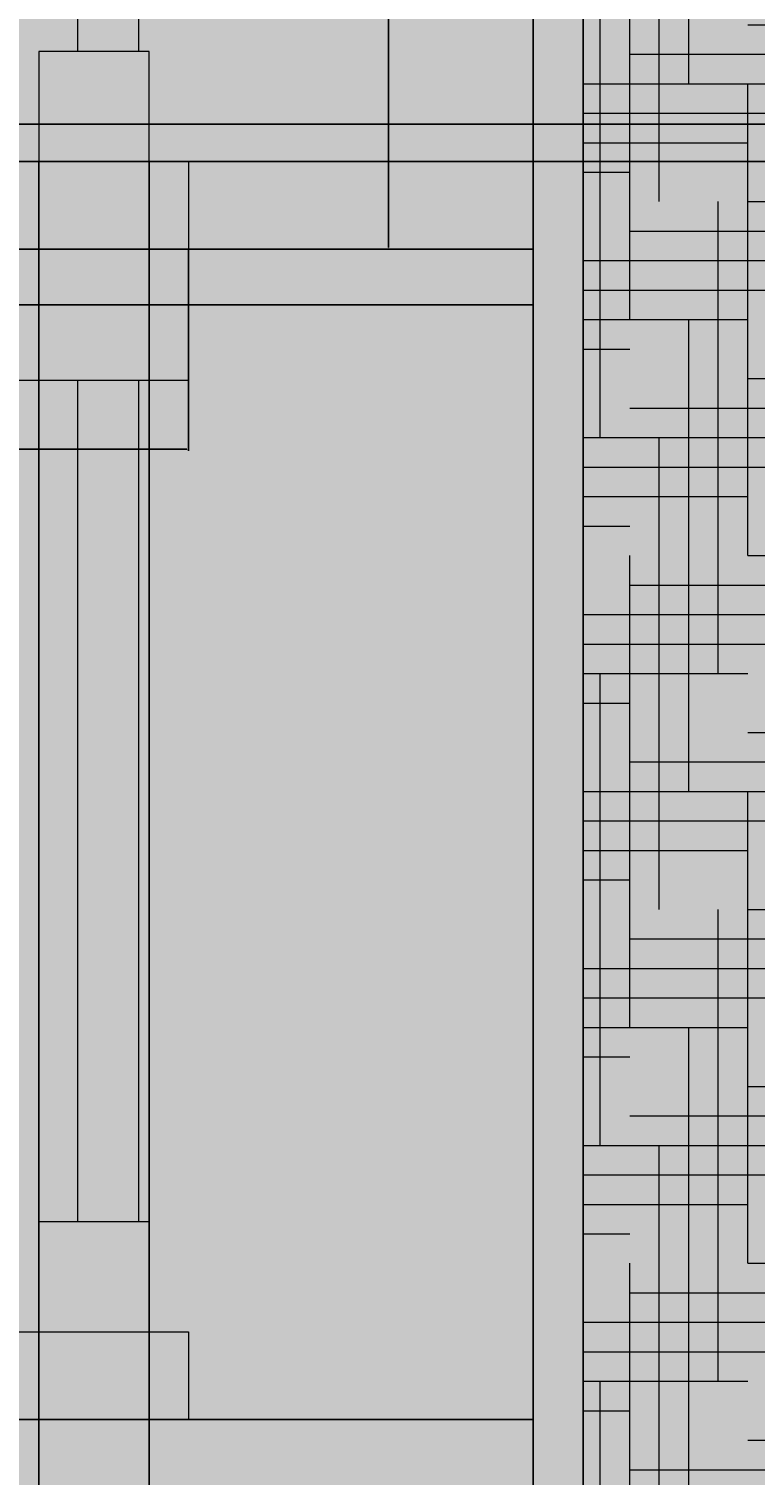
# Model space of a CAD drawing. Units: inches. Extents: x 3024 to 4744, y 1110 to 2100.
# Tile 22 of 29: x 3275 to 3354, y 1654 to 1809. Entities that reach past the tile are written whole.
import ezdxf

# ---------------------------------------------------------------- set-up
doc = ezdxf.new("R2010")
doc.units = ezdxf.units.IN
for name, color, linetype, lineweight in [('A-ANNO-DIMS', 2, 'Continuous', 18), ('A-ELEV', 7, 'Continuous', 25), ('A-ELEV-PATT', 252, 'Continuous', 13), ('A-GLAZ', 4, 'Continuous', 18)]:
    doc.layers.add(name, color=color, linetype=linetype, lineweight=lineweight)
doc.styles.get("Standard").update_dxf_attribs({"font": 'arial.ttf'})
doc.dimstyles.get("Standard").update_dxf_attribs({"dimtxt": 0.18, "dimasz": 0.18, "dimexe": 0.18, "dimexo": 0.0625, "dimgap": 0.09, "dimtad": 0, "dimtih": 1, "dimtoh": 1, "dimdec": 1, "dimzin": 0, "dimdsep": 46, "dimlunit": 3, "dimtxsty": 'Standard', "dimcen": 0.09, "dimadec": 0, "dimazin": 0, "dimtfac": 1, "dimtdec": 1, "dimtofl": 0, "dimtmove": 0, "dimatfit": 3, "dimfxl": 1, "dimtolj": 1, "dimtzin": 0, "dimarcsym": 0})

# ---------------------------------------------------------------- blocks, each defined once
blk = doc.blocks.new('WIN-BALCONY-A')
for p, q in [((3169.4, 1897.49), (3148.97, 1897.49)), ((3169.4, 1897.49), (3148.97, 1897.49)), ((3169.4, 1897.49), (3292.61, 1897.49)), ((3169.4, 1897.49), (3292.61, 1897.49)), ((3169.4, 1795.04), (3148.97, 1795.04)), ((3169.4, 1795.04), (3148.97, 1795.04)), ((3169.4, 1795.04), (3292.61, 1795.04)), ((3169.4, 1795.04), (3292.61, 1795.04))]:
    blk.add_line(p, q)
for points in [[(3148.97, 1897.49), (3148.97, 1905.61), (3292.61, 1905.61), (3292.61, 1897.49)], [(3148.97, 1897.49), (3148.97, 1905.61), (3292.61, 1905.61), (3292.61, 1897.49)], [(3292.61, 1795.04), (3292.61, 1785.61), (3148.97, 1785.61), (3148.97, 1795.04)], [(3292.61, 1795.04), (3292.61, 1785.61), (3148.97, 1785.61), (3148.97, 1795.04)]]:
    blk.add_lwpolyline(points)
for points in [[(3154.33, 1806.87), (3160.86, 1806.87), (3160.86, 1897.49), (3154.33, 1897.49)], [(3154.33, 1806.87), (3160.86, 1806.87), (3160.86, 1897.49), (3154.33, 1897.49)], [(3272.18, 1795.04), (3169.4, 1795.04), (3169.4, 1897.49), (3272.18, 1897.49)], [(3272.18, 1795.04), (3169.4, 1795.04), (3169.4, 1897.49), (3272.18, 1897.49)], [(3287.25, 1806.87), (3280.72, 1806.87), (3280.72, 1897.49), (3287.25, 1897.49)], [(3287.25, 1806.87), (3280.72, 1806.87), (3280.72, 1897.49), (3287.25, 1897.49)], [(3268.18, 1799.04), (3173.4, 1799.04), (3173.4, 1893.49), (3268.18, 1893.49)], [(3268.18, 1799.04), (3173.4, 1799.04), (3173.4, 1893.49), (3268.18, 1893.49)], [(3220.05, 1893.49), (3221.52, 1893.49), (3221.52, 1799.04), (3220.05, 1799.04)], [(3220.05, 1893.49), (3221.52, 1893.49), (3221.52, 1799.04), (3220.05, 1799.04)], [(3163.53, 1795.04), (3151.66, 1795.04), (3151.66, 1806.87), (3163.53, 1806.87)], [(3163.53, 1795.04), (3151.66, 1795.04), (3151.66, 1806.87), (3163.53, 1806.87)], [(3276.51, 1795.04), (3288.38, 1795.04), (3288.38, 1806.87), (3276.51, 1806.87)], [(3276.51, 1795.04), (3288.38, 1795.04), (3288.38, 1806.87), (3276.51, 1806.87)]]:
    blk.add_lwpolyline(points, close=True)
blk = doc.blocks.new('*D6')
at = {"layer": 'A-ANNO-DIMS', "color": 0, "lineweight": -2, "transparency": 16777216}
for p, q in [((3148.97, 1785.55), (3148.97, 1763.89)), ((3292.61, 1785.55), (3292.61, 1763.89)), ((3149.15, 1764.07), (3218.85, 1764.07)), ((3292.43, 1764.07), (3222.72, 1764.07))]:
    blk.add_line(p, q, dxfattribs=at)
at = {"layer": 'A-ANNO-DIMS', "color": 0, "transparency": 16777216}
for points in [[(3149.15, 1764.1), (3149.15, 1764.04), (3148.97, 1764.07)], [(3292.43, 1764.1), (3292.43, 1764.04), (3292.61, 1764.07)]]:
    blk.add_solid(points, dxfattribs=at)
at = {"layer": 'Defpoints', "color": 0, "transparency": 16777216}
for p in [(3148.97, 1785.61), (3292.61, 1785.61), (3292.61, 1764.07)]:
    blk.add_point(p, dxfattribs=at)
at = {"layer": 'A-ANNO-DIMS', "color": 0, "transparency": 16777216, "insert": (3220.79, 1764.07), "char_height": 0.18, "attachment_point": 5}
blk.add_mtext('\\A1;BALCONY WINDOW A 144 TYP.', dxfattribs=at)
blk = doc.blocks.new('*D7')
at = {"layer": 'A-ANNO-DIMS', "color": 0, "lineweight": -2, "transparency": 16777216}
for p, q in [((3292.67, 1905.61), (3314.33, 1905.61)), ((3314.15, 1905.43), (3314.15, 1845.79)), ((3314.15, 1785.79), (3314.15, 1845.43)), ((3292.67, 1785.61), (3314.33, 1785.61))]:
    blk.add_line(p, q, dxfattribs=at)
at = {"layer": 'A-ANNO-DIMS', "color": 0, "transparency": 16777216}
for points in [[(3314.12, 1905.43), (3314.18, 1905.43), (3314.15, 1905.61)], [(3314.12, 1785.79), (3314.18, 1785.79), (3314.15, 1785.61)]]:
    blk.add_solid(points, dxfattribs=at)
at = {"layer": 'Defpoints', "color": 0, "transparency": 16777216}
for p in [(3292.61, 1905.61), (3314.15, 1905.61), (3292.61, 1785.61)]:
    blk.add_point(p, dxfattribs=at)
at = {"layer": 'A-ANNO-DIMS', "color": 0, "transparency": 16777216, "insert": (3314.15, 1845.61), "char_height": 0.18, "attachment_point": 5}
blk.add_mtext('\\A1;120 TYP.', dxfattribs=at)
blk = doc.blocks.new('*D64')
at = {"layer": 'A-ANNO-DIMS', "color": 0, "lineweight": -2, "transparency": 16777216}
for p, q in [((3069.79, 1241.5), (3069.79, 2100.44)), ((3741.15, 1241.5), (3741.15, 2100.44)), ((3069.97, 2100.26), (3405.08, 2100.26)), ((3740.97, 2100.26), (3405.87, 2100.26))]:
    blk.add_line(p, q, dxfattribs=at)
at = {"layer": 'A-ANNO-DIMS', "color": 0, "transparency": 16777216}
for points in [[(3069.97, 2100.29), (3069.97, 2100.23), (3069.79, 2100.26)], [(3740.97, 2100.29), (3740.97, 2100.23), (3741.15, 2100.26)]]:
    blk.add_solid(points, dxfattribs=at)
at = {"layer": 'Defpoints', "color": 0, "transparency": 16777216}
for p in [(3741.15, 2100.26), (3069.79, 1241.43), (3741.15, 1241.43)]:
    blk.add_point(p, dxfattribs=at)
at = {"layer": 'A-ANNO-DIMS', "color": 0, "transparency": 16777216, "insert": (3405.47, 2100.26), "char_height": 0.18, "attachment_point": 5}
blk.add_mtext('\\A1;671.4', dxfattribs=at)
blk = doc.blocks.new('*D94')
at = {"layer": 'A-ANNO-DIMS', "color": 0, "lineweight": -2, "transparency": 16777216}
for p, q in [((3276.51, 1794.98), (3276.51, 1109.93)), ((3288.38, 1794.98), (3288.38, 1109.93)), ((3276.69, 1110.11), (3281.99, 1110.11)), ((3288.2, 1110.11), (3282.9, 1110.11))]:
    blk.add_line(p, q, dxfattribs=at)
at = {"layer": 'A-ANNO-DIMS', "color": 0, "transparency": 16777216}
for points in [[(3276.69, 1110.14), (3276.69, 1110.08), (3276.51, 1110.11)], [(3288.2, 1110.14), (3288.2, 1110.08), (3288.38, 1110.11)]]:
    blk.add_solid(points, dxfattribs=at)
at = {"layer": 'Defpoints', "color": 0, "transparency": 16777216}
for p in [(3276.51, 1795.04), (3288.38, 1795.04), (3288.38, 1110.11)]:
    blk.add_point(p, dxfattribs=at)
at = {"layer": 'A-ANNO-DIMS', "color": 0, "transparency": 16777216, "insert": (3282.44, 1110.11), "char_height": 0.18, "attachment_point": 5}
blk.add_mtext('\\A1;11.866', dxfattribs=at)
blk = doc.blocks.new('*D100')
at = {"layer": 'A-ANNO-DIMS', "color": 0, "lineweight": -2, "transparency": 16777216}
for p, q in [((3268.24, 1799.04), (3786.83, 1799.04)), ((3786.65, 1798.86), (3786.65, 1797.23)), ((3786.65, 1795.22), (3786.65, 1796.86)), ((3272.24, 1795.04), (3786.83, 1795.04))]:
    blk.add_line(p, q, dxfattribs=at)
at = {"layer": 'A-ANNO-DIMS', "color": 0, "transparency": 16777216}
for points in [[(3786.62, 1798.86), (3786.68, 1798.86), (3786.65, 1799.04)], [(3786.62, 1795.22), (3786.68, 1795.22), (3786.65, 1795.04)]]:
    blk.add_solid(points, dxfattribs=at)
at = {"layer": 'Defpoints', "color": 0, "transparency": 16777216}
for p in [(3268.18, 1799.04), (3786.65, 1799.04), (3272.18, 1795.04)]:
    blk.add_point(p, dxfattribs=at)
at = {"layer": 'A-ANNO-DIMS', "color": 0, "transparency": 16777216, "insert": (3786.65, 1797.04), "char_height": 0.18, "attachment_point": 5}
blk.add_mtext('\\A1;4.00', dxfattribs=at)
blk = doc.blocks.new('*D101')
at = {"layer": 'A-ANNO-DIMS', "color": 0, "lineweight": -2, "transparency": 16777216}
for p, q in [((3268.24, 1893.49), (3786.83, 1893.49)), ((3786.65, 1893.31), (3786.65, 1846.45)), ((3786.65, 1799.22), (3786.65, 1846.08)), ((3268.24, 1799.04), (3786.83, 1799.04))]:
    blk.add_line(p, q, dxfattribs=at)
at = {"layer": 'A-ANNO-DIMS', "color": 0, "transparency": 16777216}
for points in [[(3786.62, 1893.31), (3786.68, 1893.31), (3786.65, 1893.49)], [(3786.62, 1799.22), (3786.68, 1799.22), (3786.65, 1799.04)]]:
    blk.add_solid(points, dxfattribs=at)
at = {"layer": 'Defpoints', "color": 0, "transparency": 16777216}
for p in [(3268.18, 1893.49), (3786.65, 1893.49), (3268.18, 1799.04)]:
    blk.add_point(p, dxfattribs=at)
at = {"layer": 'A-ANNO-DIMS', "color": 0, "transparency": 16777216, "insert": (3786.65, 1846.27), "char_height": 0.18, "attachment_point": 5}
blk.add_mtext('\\A1;94.44', dxfattribs=at)

msp = doc.modelspace()

# ---------------------------------------------------------------- hatches: boundary and pattern name
at = {"layer": 'A-ELEV-PATT'}
h = msp.add_hatch(color=256, dxfattribs=at)
h.dxf.hatch_style = 1
h.paths.add_polyline_path([(3491.8271, 2054.7584), (3320.5658, 2054.7584), (3320.5658, 2043.5286), (3491.8271, 2043.5286)])
h.paths.add_polyline_path([(3292.6051, 1905.6112), (3148.9694, 1905.6112), (3148.9694, 1897.4879), (3169.3964, 1897.4879), (3292.6051, 1897.4879)])
h.paths.add_polyline_path([(3292.6051, 1795.0431), (3169.3964, 1795.0431), (3148.9694, 1795.0431), (3148.9694, 1785.6112), (3292.6051, 1785.6112)])
h.paths.add_polyline_path([(3292.6051, 1779.6112), (3148.9694, 1779.6112), (3148.9694, 1771.4879), (3169.3964, 1771.4879), (3292.6051, 1771.4879)])
h.paths.add_polyline_path([(3292.6051, 1669.0431), (3169.3964, 1669.0431), (3148.9694, 1669.0431), (3148.9694, 1659.6112), (3292.6051, 1659.6112)])
h.paths.add_polyline_path([(3292.6051, 1653.6112), (3148.9694, 1653.6112), (3148.9694, 1645.4879), (3169.3964, 1645.4879), (3292.6051, 1645.4879)])
h.paths.add_polyline_path([(3292.6051, 1543.0431), (3169.3964, 1543.0431), (3148.9694, 1543.0431), (3148.9694, 1533.6112), (3292.6051, 1533.6112)])
h.paths.add_polyline_path([(3292.6051, 1527.6112), (3148.9694, 1527.6112), (3148.9694, 1519.4879), (3169.3964, 1519.4879), (3292.6051, 1519.4879)])
h.paths.add_polyline_path([(3292.6051, 1401.6112), (3148.9694, 1401.6112), (3148.9694, 1393.4879), (3169.3964, 1393.4879), (3292.6051, 1393.4879)])
h.paths.add_polyline_path([(3292.6051, 1417.0431), (3169.3964, 1417.0431), (3148.9694, 1417.0431), (3148.9694, 1407.6112), (3292.6051, 1407.6112)])
h.paths.add_polyline_path([(3292.6051, 1291.0431), (3169.3964, 1291.0431), (3148.9694, 1291.0431), (3148.9694, 1281.6112), (3292.6051, 1281.6112)])
h.paths.add_polyline_path([(3654.037, 1165.0431), (3530.8283, 1165.0431), (3510.4013, 1165.0431), (3510.4013, 1155.6112), (3654.037, 1155.6112)])
h.paths.add_polyline_path([(3654.037, 1275.6112), (3510.4013, 1275.6112), (3510.4013, 1267.4879), (3530.8283, 1267.4879), (3654.037, 1267.4879)])
h.paths.add_polyline_path([(3654.037, 1291.0431), (3530.8283, 1291.0431), (3510.4013, 1291.0431), (3510.4013, 1281.6112), (3654.037, 1281.6112)])
h.paths.add_polyline_path([(3654.037, 1417.0431), (3530.8283, 1417.0431), (3510.4013, 1417.0431), (3510.4013, 1407.6112), (3654.037, 1407.6112)])
h.paths.add_polyline_path([(3654.037, 1401.6112), (3510.4013, 1401.6112), (3510.4013, 1393.4879), (3530.8283, 1393.4879), (3654.037, 1393.4879)])
h.paths.add_polyline_path([(3654.037, 1543.0431), (3530.8283, 1543.0431), (3510.4013, 1543.0431), (3510.4013, 1533.6112), (3654.037, 1533.6112)])
h.paths.add_polyline_path([(3654.037, 1527.6112), (3510.4013, 1527.6112), (3510.4013, 1519.4879), (3530.8283, 1519.4879), (3654.037, 1519.4879)])
h.paths.add_polyline_path([(3654.037, 1653.6112), (3510.4013, 1653.6112), (3510.4013, 1645.4879), (3530.8283, 1645.4879), (3654.037, 1645.4879)])
h.paths.add_polyline_path([(3654.037, 1669.0431), (3530.8283, 1669.0431), (3510.4013, 1669.0431), (3510.4013, 1659.6112), (3654.037, 1659.6112)])
h.paths.add_polyline_path([(3654.037, 1779.6112), (3510.4013, 1779.6112), (3510.4013, 1771.4879), (3530.8283, 1771.4879), (3654.037, 1771.4879)])
h.paths.add_polyline_path([(3654.037, 1795.0431), (3530.8283, 1795.0431), (3510.4013, 1795.0431), (3510.4013, 1785.6112), (3654.037, 1785.6112)])
h.paths.add_polyline_path([(3654.037, 1905.6112), (3510.4013, 1905.6112), (3510.4013, 1897.4879), (3530.8283, 1897.4879), (3654.037, 1897.4879)])
h = msp.add_hatch(color=256, dxfattribs=at)
h.dxf.hatch_style = 1
h.paths.add_polyline_path([(3335.1044, 2043.5286), (3329.7033, 2043.5286), (3329.7033, 1155.6112), (3335.1044, 1155.6112)])
h.paths.add_polyline_path([(3481.2411, 2043.5286), (3335.1044, 2043.5286), (3335.1044, 1155.6112), (3481.2411, 1155.6112)])
h.paths.add_polyline_path([(3449.7202, 1329.5246), (3361.2242, 1329.5246), (3361.2242, 1436.6064), (3449.7202, 1436.6064)], flags=16)
h.paths.add_polyline_path([(3445.7202, 1333.5246), (3365.2242, 1333.5246), (3365.2242, 1432.6064), (3445.7202, 1432.6064)], flags=0)
h.paths.add_polyline_path([(3449.7202, 1455.5246), (3361.2242, 1455.5246), (3361.2242, 1562.6064), (3449.7202, 1562.6064)], flags=16)
h.paths.add_polyline_path([(3445.7202, 1459.5246), (3365.2242, 1459.5246), (3365.2242, 1558.6064), (3445.7202, 1558.6064)], flags=0)
h.paths.add_polyline_path([(3449.7202, 1581.5246), (3361.2242, 1581.5246), (3361.2242, 1688.6064), (3449.7202, 1688.6064)], flags=16)
h.paths.add_polyline_path([(3445.7202, 1585.5246), (3365.2242, 1585.5246), (3365.2242, 1684.6064), (3445.7202, 1684.6064)], flags=0)
h.paths.add_polyline_path([(3449.7202, 1707.5246), (3361.2242, 1707.5246), (3361.2242, 1814.6064), (3449.7202, 1814.6064)], flags=16)
h.paths.add_polyline_path([(3445.7202, 1711.5246), (3365.2242, 1711.5246), (3365.2242, 1810.6064), (3445.7202, 1810.6064)], flags=0)
h.paths.add_polyline_path([(3449.7202, 1833.5246), (3361.2242, 1833.5246), (3361.2242, 1940.6064), (3449.7202, 1940.6064)], flags=16)
h.paths.add_polyline_path([(3445.7202, 1837.5246), (3365.2242, 1837.5246), (3365.2242, 1936.6064), (3445.7202, 1936.6064)], flags=0)
h = msp.add_hatch(color=256, dxfattribs=at)
h.dxf.hatch_style = 1
h.paths.add_polyline_path([(3475.84, 2043.5286), (3335.1044, 2043.5286), (3335.1044, 1155.6112), (3475.84, 1155.6112)])
h.paths.add_polyline_path([(3449.7202, 1940.6064), (3449.7202, 1833.5246), (3361.2242, 1833.5246), (3361.2242, 1940.6064)], flags=16)
h.paths.add_polyline_path([(3445.7202, 1936.6064), (3445.7202, 1837.5246), (3365.2242, 1837.5246), (3365.2242, 1936.6064)], flags=0)
h.paths.add_polyline_path([(3449.7202, 1814.6064), (3449.7202, 1707.5246), (3361.2242, 1707.5246), (3361.2242, 1814.6064)], flags=16)
h.paths.add_polyline_path([(3445.7202, 1810.6064), (3445.7202, 1711.5246), (3365.2242, 1711.5246), (3365.2242, 1810.6064)], flags=0)
h.paths.add_polyline_path([(3449.7202, 1688.6064), (3449.7202, 1581.5246), (3361.2242, 1581.5246), (3361.2242, 1688.6064)], flags=16)
h.paths.add_polyline_path([(3445.7202, 1684.6064), (3445.7202, 1585.5246), (3365.2242, 1585.5246), (3365.2242, 1684.6064)], flags=0)
h.paths.add_polyline_path([(3449.7202, 1562.6064), (3449.7202, 1455.5246), (3361.2242, 1455.5246), (3361.2242, 1562.6064)], flags=16)
h.paths.add_polyline_path([(3445.7202, 1558.6064), (3445.7202, 1459.5246), (3365.2242, 1459.5246), (3365.2242, 1558.6064)], flags=0)
h.paths.add_polyline_path([(3449.7202, 1436.6064), (3449.7202, 1329.5246), (3361.2242, 1329.5246), (3361.2242, 1436.6064)], flags=16)
h.paths.add_polyline_path([(3445.7202, 1432.6064), (3445.7202, 1333.5246), (3365.2242, 1333.5246), (3365.2242, 1432.6064)], flags=0)
h = msp.add_hatch(dxfattribs=at)
h.set_pattern_fill('HOUND', color=256, scale=2)
h.paths.add_polyline_path([(3475.84, 2043.5286), (3335.1044, 2043.5286), (3335.1044, 1155.6112), (3475.84, 1155.6112)])
h.paths.add_polyline_path([(3449.7202, 1940.6064), (3449.7202, 1833.5246), (3361.2242, 1833.5246), (3361.2242, 1940.6064)], flags=16)
h.paths.add_polyline_path([(3445.7202, 1936.6064), (3445.7202, 1837.5246), (3365.2242, 1837.5246), (3365.2242, 1936.6064)], flags=0)
h.paths.add_polyline_path([(3449.7202, 1814.6064), (3449.7202, 1707.5246), (3361.2242, 1707.5246), (3361.2242, 1814.6064)], flags=16)
h.paths.add_polyline_path([(3445.7202, 1810.6064), (3445.7202, 1711.5246), (3365.2242, 1711.5246), (3365.2242, 1810.6064)], flags=0)
h.paths.add_polyline_path([(3449.7202, 1688.6064), (3449.7202, 1581.5246), (3361.2242, 1581.5246), (3361.2242, 1688.6064)], flags=16)
h.paths.add_polyline_path([(3445.7202, 1684.6064), (3445.7202, 1585.5246), (3365.2242, 1585.5246), (3365.2242, 1684.6064)], flags=0)
h.paths.add_polyline_path([(3449.7202, 1562.6064), (3449.7202, 1455.5246), (3361.2242, 1455.5246), (3361.2242, 1562.6064)], flags=16)
h.paths.add_polyline_path([(3445.7202, 1558.6064), (3445.7202, 1459.5246), (3365.2242, 1459.5246), (3365.2242, 1558.6064)], flags=0)
h.paths.add_polyline_path([(3449.7202, 1436.6064), (3449.7202, 1329.5246), (3361.2242, 1329.5246), (3361.2242, 1436.6064)], flags=16)
h.paths.add_polyline_path([(3445.7202, 1432.6064), (3445.7202, 1333.5246), (3365.2242, 1333.5246), (3365.2242, 1432.6064)], flags=0)
h = msp.add_hatch(color=256, dxfattribs=at)
h.dxf.hatch_style = 1
h.paths.add_polyline_path([(3329.7033, 1407.6112), (3105.4722, 1407.6112), (3105.4722, 1401.6112), (3329.7033, 1401.6112)])
h.paths.add_polyline_path([(3329.7033, 1281.6112), (3105.4722, 1281.6112), (3105.4722, 1275.6112), (3112.3838, 1275.6112), (3329.7033, 1275.6112)])
h.paths.add_polyline_path([(3329.7033, 1533.6112), (3105.4722, 1533.6112), (3105.4722, 1527.6112), (3329.7033, 1527.6112)])
h.paths.add_polyline_path([(3329.7033, 1659.6112), (3105.4722, 1659.6112), (3105.4722, 1653.6112), (3329.7033, 1653.6112)])
h.paths.add_polyline_path([(3329.7033, 1785.6112), (3105.4722, 1785.6112), (3105.4722, 1779.6112), (3329.7033, 1779.6112)])
h.paths.add_polyline_path([(3329.7033, 1911.6112), (3105.4722, 1911.6112), (3095.7158, 1911.6112), (3095.7158, 1905.6112), (3329.7033, 1905.6112)])
h.paths.add_polyline_path([(3715.2286, 1911.6112), (3705.4722, 1911.6112), (3705.4722, 1905.6112), (3715.2286, 1905.6112)])
h.paths.add_polyline_path([(3688.5588, 1911.6112), (3481.2411, 1911.6112), (3481.2411, 1905.6112), (3688.5588, 1905.6112)])
h = msp.add_hatch(color=256, dxfattribs=at)
h.dxf.hatch_style = 1
h.paths.add_polyline_path([(3154.3287, 1897.4879), (3148.9694, 1897.4879), (3148.9694, 1905.6112), (3105.4722, 1905.6112), (3105.4722, 1785.6112), (3148.9694, 1785.6112), (3148.9694, 1795.0431), (3151.6604, 1795.0431), (3151.6604, 1806.8674), (3154.3287, 1806.8674)])
h.paths.add_polyline_path([(3329.7033, 1905.6112), (3292.6051, 1905.6112), (3292.6051, 1897.4879), (3287.2458, 1897.4879), (3287.2458, 1806.8674), (3288.3759, 1806.8674), (3288.3759, 1795.0431), (3292.6051, 1795.0431), (3292.6051, 1785.6112), (3329.7033, 1785.6112)])
h.paths.add_polyline_path([(3154.3287, 1771.4879), (3148.9694, 1771.4879), (3148.9694, 1779.6112), (3105.4722, 1779.6112), (3105.4722, 1659.6112), (3148.9694, 1659.6112), (3148.9694, 1669.0431), (3151.6604, 1669.0431), (3151.6604, 1680.8674), (3154.3287, 1680.8674)])
h.paths.add_polyline_path([(3329.7033, 1779.6112), (3292.6051, 1779.6112), (3292.6051, 1771.4879), (3287.2458, 1771.4879), (3287.2458, 1680.8674), (3288.3759, 1680.8674), (3288.3759, 1669.0431), (3292.6051, 1669.0431), (3292.6051, 1659.6112), (3329.7033, 1659.6112)])
h.paths.add_polyline_path([(3154.3287, 1645.4879), (3148.9694, 1645.4879), (3148.9694, 1653.6112), (3105.4722, 1653.6112), (3105.4722, 1533.6112), (3148.9694, 1533.6112), (3148.9694, 1543.0431), (3151.6604, 1543.0431), (3151.6604, 1554.8674), (3154.3287, 1554.8674)])
h.paths.add_polyline_path([(3329.7033, 1653.6112), (3292.6051, 1653.6112), (3292.6051, 1645.4879), (3287.2458, 1645.4879), (3287.2458, 1554.8674), (3288.3759, 1554.8674), (3288.3759, 1543.0431), (3292.6051, 1543.0431), (3292.6051, 1533.6112), (3329.7033, 1533.6112)])
h.paths.add_polyline_path([(3329.7033, 1527.6112), (3292.6051, 1527.6112), (3292.6051, 1519.4879), (3287.2458, 1519.4879), (3287.2458, 1428.8674), (3288.3759, 1428.8674), (3288.3759, 1417.0431), (3292.6051, 1417.0431), (3292.6051, 1407.6112), (3329.7033, 1407.6112)])
h.paths.add_polyline_path([(3329.7033, 1401.6112), (3292.6051, 1401.6112), (3292.6051, 1393.4879), (3287.2458, 1393.4879), (3287.2458, 1302.8674), (3288.3759, 1302.8674), (3288.3759, 1291.0431), (3292.6051, 1291.0431), (3292.6051, 1281.6112), (3329.7033, 1281.6112)])
h.paths.add_polyline_path([(3154.3287, 1393.4879), (3148.9694, 1393.4879), (3148.9694, 1401.6112), (3105.4722, 1401.6112), (3105.4722, 1281.6112), (3148.9694, 1281.6112), (3148.9694, 1291.0431), (3151.6604, 1291.0431), (3151.6604, 1302.8674), (3154.3287, 1302.8674)])
h.paths.add_polyline_path([(3154.3287, 1519.4879), (3148.9694, 1519.4879), (3148.9694, 1527.6112), (3105.4722, 1527.6112), (3105.4722, 1407.6112), (3148.9694, 1407.6112), (3148.9694, 1417.0431), (3151.6604, 1417.0431), (3151.6604, 1428.8674), (3154.3287, 1428.8674)])
h.paths.add_polyline_path([(3515.7606, 1897.4879), (3510.4013, 1897.4879), (3510.4013, 1905.6112), (3481.2411, 1905.6112), (3481.2411, 1785.6112), (3510.4013, 1785.6112), (3510.4013, 1795.0431), (3513.0923, 1795.0431), (3513.0923, 1806.8674), (3515.7606, 1806.8674)])
h.paths.add_polyline_path([(3688.5588, 1905.6112), (3654.037, 1905.6112), (3654.037, 1897.4879), (3648.6777, 1897.4879), (3648.6777, 1806.8674), (3649.8078, 1806.8674), (3649.8078, 1795.0431), (3654.037, 1795.0431), (3654.037, 1785.6112), (3688.5588, 1785.6112)])
h.paths.add_polyline_path([(3515.7606, 1771.4879), (3510.4013, 1771.4879), (3510.4013, 1779.6112), (3481.2411, 1779.6112), (3481.2411, 1659.6112), (3510.4013, 1659.6112), (3510.4013, 1669.0431), (3513.0923, 1669.0431), (3513.0923, 1680.8674), (3515.7606, 1680.8674)])
h.paths.add_polyline_path([(3688.5588, 1779.6112), (3654.037, 1779.6112), (3654.037, 1771.4879), (3648.6777, 1771.4879), (3648.6777, 1680.8674), (3649.8078, 1680.8674), (3649.8078, 1669.0431), (3654.037, 1669.0431), (3654.037, 1659.6112), (3688.5588, 1659.6112)])
h.paths.add_polyline_path([(3515.7606, 1645.4879), (3510.4013, 1645.4879), (3510.4013, 1653.6112), (3481.2411, 1653.6112), (3481.2411, 1533.6112), (3510.4013, 1533.6112), (3510.4013, 1543.0431), (3513.0923, 1543.0431), (3513.0923, 1554.8674), (3515.7606, 1554.8674)])
h.paths.add_polyline_path([(3688.5588, 1653.6112), (3654.037, 1653.6112), (3654.037, 1645.4879), (3648.6777, 1645.4879), (3648.6777, 1554.8674), (3649.8078, 1554.8674), (3649.8078, 1543.0431), (3654.037, 1543.0431), (3654.037, 1533.6112), (3688.5588, 1533.6112)])
h.paths.add_polyline_path([(3515.7606, 1519.4879), (3510.4013, 1519.4879), (3510.4013, 1527.6112), (3481.2411, 1527.6112), (3481.2411, 1407.6112), (3510.4013, 1407.6112), (3510.4013, 1417.0431), (3513.0923, 1417.0431), (3513.0923, 1428.8674), (3515.7606, 1428.8674)])
h.paths.add_polyline_path([(3688.5588, 1527.6112), (3654.037, 1527.6112), (3654.037, 1519.4879), (3648.6777, 1519.4879), (3648.6777, 1428.8674), (3649.8078, 1428.8674), (3649.8078, 1417.0431), (3654.037, 1417.0431), (3654.037, 1407.6112), (3688.5588, 1407.6112)])
h.paths.add_polyline_path([(3515.7606, 1393.4879), (3510.4013, 1393.4879), (3510.4013, 1401.6112), (3481.2411, 1401.6112), (3481.2411, 1281.6112), (3510.4013, 1281.6112), (3510.4013, 1291.0431), (3513.0923, 1291.0431), (3513.0923, 1302.8674), (3515.7606, 1302.8674)])
h.paths.add_polyline_path([(3688.5588, 1401.6112), (3654.037, 1401.6112), (3654.037, 1393.4879), (3648.6777, 1393.4879), (3648.6777, 1302.8674), (3649.8078, 1302.8674), (3649.8078, 1291.0431), (3654.037, 1291.0431), (3654.037, 1281.6112), (3688.5588, 1281.6112)])
h.paths.add_polyline_path([(3515.7606, 1267.4879), (3510.4013, 1267.4879), (3510.4013, 1275.6112), (3481.2411, 1275.6112), (3481.2411, 1155.6112), (3510.4013, 1155.6112), (3510.4013, 1165.0431), (3513.0923, 1165.0431), (3513.0923, 1176.8674), (3515.7606, 1176.8674)])
h.paths.add_polyline_path([(3688.5588, 1275.6112), (3654.037, 1275.6112), (3654.037, 1267.4879), (3648.6777, 1267.4879), (3648.6777, 1176.8674), (3649.8078, 1176.8674), (3649.8078, 1165.0431), (3654.037, 1165.0431), (3654.037, 1155.6112), (3688.5588, 1155.6112)])
h.paths.add_polyline_path([(3112.3838, 1275.6112), (3105.4722, 1275.6112), (3105.4722, 1171.0239), (3112.3838, 1171.0239)])
h = msp.add_hatch(color=256, dxfattribs=at)
h.dxf.hatch_style = 1
h.paths.add_polyline_path([(3160.8586, 1897.4879), (3154.3287, 1897.4879), (3154.3287, 1806.8674), (3160.8586, 1806.8674)])
h.paths.add_polyline_path([(3287.2458, 1897.4879), (3280.716, 1897.4879), (3280.716, 1806.8674), (3287.2458, 1806.8674)])
h.paths.add_polyline_path([(3160.8586, 1771.4879), (3154.3287, 1771.4879), (3154.3287, 1680.8674), (3160.8586, 1680.8674)])
h.paths.add_polyline_path([(3287.2458, 1771.4879), (3280.716, 1771.4879), (3280.716, 1680.8674), (3287.2458, 1680.8674)])
h.paths.add_polyline_path([(3160.8586, 1645.4879), (3154.3287, 1645.4879), (3154.3287, 1554.8674), (3160.8586, 1554.8674)])
h.paths.add_polyline_path([(3287.2458, 1645.4879), (3280.716, 1645.4879), (3280.716, 1554.8674), (3287.2458, 1554.8674)])
h.paths.add_polyline_path([(3160.8586, 1519.4879), (3154.3287, 1519.4879), (3154.3287, 1428.8674), (3160.8586, 1428.8674)])
h.paths.add_polyline_path([(3287.2458, 1519.4879), (3280.716, 1519.4879), (3280.716, 1428.8674), (3287.2458, 1428.8674)])
h.paths.add_polyline_path([(3160.8586, 1393.4879), (3154.3287, 1393.4879), (3154.3287, 1302.8674), (3160.8586, 1302.8674)])
h.paths.add_polyline_path([(3287.2458, 1393.4879), (3280.716, 1393.4879), (3280.716, 1302.8674), (3287.2458, 1302.8674)])
h.paths.add_polyline_path([(3648.6777, 1267.4879), (3642.1479, 1267.4879), (3642.1479, 1176.8674), (3648.6777, 1176.8674)])
h.paths.add_polyline_path([(3522.2905, 1267.4879), (3515.7606, 1267.4879), (3515.7606, 1176.8674), (3522.2905, 1176.8674)])
h.paths.add_polyline_path([(3522.2905, 1393.4879), (3515.7606, 1393.4879), (3515.7606, 1302.8674), (3522.2905, 1302.8674)])
h.paths.add_polyline_path([(3648.6777, 1393.4879), (3642.1479, 1393.4879), (3642.1479, 1302.8674), (3648.6777, 1302.8674)])
h.paths.add_polyline_path([(3522.2905, 1519.4879), (3515.7606, 1519.4879), (3515.7606, 1428.8674), (3522.2905, 1428.8674)])
h.paths.add_polyline_path([(3648.6777, 1519.4879), (3642.1479, 1519.4879), (3642.1479, 1428.8674), (3648.6777, 1428.8674)])
h.paths.add_polyline_path([(3522.2905, 1645.4879), (3515.7606, 1645.4879), (3515.7606, 1554.8674), (3522.2905, 1554.8674)])
h.paths.add_polyline_path([(3522.2905, 1771.4879), (3515.7606, 1771.4879), (3515.7606, 1680.8674), (3522.2905, 1680.8674)])
h.paths.add_polyline_path([(3648.6777, 1645.4879), (3642.1479, 1645.4879), (3642.1479, 1554.8674), (3648.6777, 1554.8674)])
h.paths.add_polyline_path([(3648.6777, 1771.4879), (3642.1479, 1771.4879), (3642.1479, 1680.8674), (3648.6777, 1680.8674)])
h.paths.add_polyline_path([(3648.6777, 1897.4879), (3642.1479, 1897.4879), (3642.1479, 1806.8674), (3648.6777, 1806.8674)])
h.paths.add_polyline_path([(3522.2905, 1897.4879), (3515.7606, 1897.4879), (3515.7606, 1806.8674), (3522.2905, 1806.8674)])
h = msp.add_hatch(color=256, dxfattribs=at)
h.dxf.hatch_style = 1
h.paths.add_polyline_path([(3169.3964, 1897.4879), (3160.8586, 1897.4879), (3160.8586, 1806.8674), (3163.5269, 1806.8674), (3163.5269, 1795.0431), (3169.3964, 1795.0431)])
h.paths.add_polyline_path([(3280.716, 1897.4879), (3272.1781, 1897.4879), (3272.1781, 1795.0431), (3276.5094, 1795.0431), (3276.5094, 1806.8674), (3280.716, 1806.8674)])
h.paths.add_polyline_path([(3280.716, 1771.4879), (3272.1781, 1771.4879), (3272.1781, 1669.0431), (3276.5094, 1669.0431), (3276.5094, 1680.8674), (3280.716, 1680.8674)])
h.paths.add_polyline_path([(3169.3964, 1771.4879), (3160.8586, 1771.4879), (3160.8586, 1680.8674), (3163.5269, 1680.8674), (3163.5269, 1669.0431), (3169.3964, 1669.0431)])
h.paths.add_polyline_path([(3169.3964, 1645.4879), (3160.8586, 1645.4879), (3160.8586, 1554.8674), (3163.5269, 1554.8674), (3163.5269, 1543.0431), (3169.3964, 1543.0431)])
h.paths.add_polyline_path([(3280.716, 1645.4879), (3272.1781, 1645.4879), (3272.1781, 1543.0431), (3276.5094, 1543.0431), (3276.5094, 1554.8674), (3280.716, 1554.8674)])
h.paths.add_polyline_path([(3169.3964, 1519.4879), (3160.8586, 1519.4879), (3160.8586, 1428.8674), (3163.5269, 1428.8674), (3163.5269, 1417.0431), (3169.3964, 1417.0431)])
h.paths.add_polyline_path([(3280.716, 1519.4879), (3272.1781, 1519.4879), (3272.1781, 1417.0431), (3276.5094, 1417.0431), (3276.5094, 1428.8674), (3280.716, 1428.8674)])
h.paths.add_polyline_path([(3169.3964, 1393.4879), (3160.8586, 1393.4879), (3160.8586, 1302.8674), (3163.5269, 1302.8674), (3163.5269, 1291.0431), (3169.3964, 1291.0431)])
h.paths.add_polyline_path([(3280.716, 1393.4879), (3272.1781, 1393.4879), (3272.1781, 1291.0431), (3276.5094, 1291.0431), (3276.5094, 1302.8674), (3280.716, 1302.8674)])
h.paths.add_polyline_path([(3642.1479, 1267.4879), (3633.61, 1267.4879), (3633.61, 1165.0431), (3637.9413, 1165.0431), (3637.9413, 1176.8674), (3642.1479, 1176.8674)])
h.paths.add_polyline_path([(3530.8283, 1267.4879), (3522.2905, 1267.4879), (3522.2905, 1176.8674), (3524.9588, 1176.8674), (3524.9588, 1165.0431), (3530.8283, 1165.0431)])
h.paths.add_polyline_path([(3642.1479, 1393.4879), (3633.61, 1393.4879), (3633.61, 1291.0431), (3637.9413, 1291.0431), (3637.9413, 1302.8674), (3642.1479, 1302.8674)])
h.paths.add_polyline_path([(3530.8283, 1393.4879), (3522.2905, 1393.4879), (3522.2905, 1302.8674), (3524.9588, 1302.8674), (3524.9588, 1291.0431), (3530.8283, 1291.0431)])
h.paths.add_polyline_path([(3530.8283, 1519.4879), (3522.2905, 1519.4879), (3522.2905, 1428.8674), (3524.9588, 1428.8674), (3524.9588, 1417.0431), (3530.8283, 1417.0431)])
h.paths.add_polyline_path([(3642.1479, 1519.4879), (3633.61, 1519.4879), (3633.61, 1417.0431), (3637.9413, 1417.0431), (3637.9413, 1428.8674), (3642.1479, 1428.8674)])
h.paths.add_polyline_path([(3530.8283, 1645.4879), (3522.2905, 1645.4879), (3522.2905, 1554.8674), (3524.9588, 1554.8674), (3524.9588, 1543.0431), (3530.8283, 1543.0431)])
h.paths.add_polyline_path([(3642.1479, 1645.4879), (3633.61, 1645.4879), (3633.61, 1543.0431), (3637.9413, 1543.0431), (3637.9413, 1554.8674), (3642.1479, 1554.8674)])
h.paths.add_polyline_path([(3642.1479, 1771.4879), (3633.61, 1771.4879), (3633.61, 1669.0431), (3637.9413, 1669.0431), (3637.9413, 1680.8674), (3642.1479, 1680.8674)])
h.paths.add_polyline_path([(3530.8283, 1771.4879), (3522.2905, 1771.4879), (3522.2905, 1680.8674), (3524.9588, 1680.8674), (3524.9588, 1669.0431), (3530.8283, 1669.0431)])
h.paths.add_polyline_path([(3530.8283, 1897.4879), (3522.2905, 1897.4879), (3522.2905, 1806.8674), (3524.9588, 1806.8674), (3524.9588, 1795.0431), (3530.8283, 1795.0431)])
h.paths.add_polyline_path([(3642.1479, 1897.4879), (3633.61, 1897.4879), (3633.61, 1795.0431), (3637.9413, 1795.0431), (3637.9413, 1806.8674), (3642.1479, 1806.8674)])
h = msp.add_hatch(color=256, dxfattribs=at)
h.dxf.hatch_style = 1
h.paths.add_polyline_path([(3163.5269, 1302.8674), (3151.6604, 1302.8674), (3151.6604, 1291.0431), (3163.5269, 1291.0431)])
h.paths.add_polyline_path([(3288.3759, 1302.8674), (3276.5094, 1302.8674), (3276.5094, 1291.0431), (3288.3759, 1291.0431)])
h.paths.add_polyline_path([(3288.3759, 1428.8674), (3276.5094, 1428.8674), (3276.5094, 1417.0431), (3288.3759, 1417.0431)])
h.paths.add_polyline_path([(3163.5269, 1428.8674), (3151.6604, 1428.8674), (3151.6604, 1417.0431), (3163.5269, 1417.0431)])
h.paths.add_polyline_path([(3163.5269, 1554.8674), (3151.6604, 1554.8674), (3151.6604, 1543.0431), (3163.5269, 1543.0431)])
h.paths.add_polyline_path([(3288.3759, 1554.8674), (3276.5094, 1554.8674), (3276.5094, 1543.0431), (3288.3759, 1543.0431)])
h.paths.add_polyline_path([(3163.5269, 1680.8674), (3151.6604, 1680.8674), (3151.6604, 1669.0431), (3163.5269, 1669.0431)])
h.paths.add_polyline_path([(3288.3759, 1680.8674), (3276.5094, 1680.8674), (3276.5094, 1669.0431), (3288.3759, 1669.0431)])
h.paths.add_polyline_path([(3163.5269, 1806.8674), (3151.6604, 1806.8674), (3151.6604, 1795.0431), (3163.5269, 1795.0431)])
h.paths.add_polyline_path([(3288.3759, 1806.8674), (3276.5094, 1806.8674), (3276.5094, 1795.0431), (3288.3759, 1795.0431)])
h.paths.add_polyline_path([(3524.9588, 1806.8674), (3513.0923, 1806.8674), (3513.0923, 1795.0431), (3524.9588, 1795.0431)])
h.paths.add_polyline_path([(3649.8078, 1806.8674), (3637.9413, 1806.8674), (3637.9413, 1795.0431), (3649.8078, 1795.0431)])
h.paths.add_polyline_path([(3524.9588, 1680.8674), (3513.0923, 1680.8674), (3513.0923, 1669.0431), (3524.9588, 1669.0431)])
h.paths.add_polyline_path([(3649.8078, 1680.8674), (3637.9413, 1680.8674), (3637.9413, 1669.0431), (3649.8078, 1669.0431)])
h.paths.add_polyline_path([(3524.9588, 1554.8674), (3513.0923, 1554.8674), (3513.0923, 1543.0431), (3524.9588, 1543.0431)])
h.paths.add_polyline_path([(3649.8078, 1554.8674), (3637.9413, 1554.8674), (3637.9413, 1543.0431), (3649.8078, 1543.0431)])
h.paths.add_polyline_path([(3524.9588, 1428.8674), (3513.0923, 1428.8674), (3513.0923, 1417.0431), (3524.9588, 1417.0431)])
h.paths.add_polyline_path([(3649.8078, 1428.8674), (3637.9413, 1428.8674), (3637.9413, 1417.0431), (3649.8078, 1417.0431)])
h.paths.add_polyline_path([(3524.9588, 1302.8674), (3513.0923, 1302.8674), (3513.0923, 1291.0431), (3524.9588, 1291.0431)])
h.paths.add_polyline_path([(3649.8078, 1302.8674), (3637.9413, 1302.8674), (3637.9413, 1291.0431), (3649.8078, 1291.0431)])
h.paths.add_polyline_path([(3524.9588, 1176.8674), (3513.0923, 1176.8674), (3513.0923, 1165.0431), (3524.9588, 1165.0431)])
h.paths.add_polyline_path([(3649.8078, 1176.8674), (3637.9413, 1176.8674), (3637.9413, 1165.0431), (3649.8078, 1165.0431)])

# ---------------------------------------------------------------- linework, layer by layer
at = {"layer": 'A-ELEV'}
for p, q in [((3105.4722, 1785.6112), (3329.7033, 1785.6112)), ((3105.4722, 1785.6112), (3329.7033, 1785.6112)), ((3329.7033, 1779.6112), (3105.4722, 1779.6112)), ((3329.7033, 1779.6112), (3105.4722, 1779.6112)), ((3105.4722, 1659.6112), (3329.7033, 1659.6112)), ((3105.4722, 1659.6112), (3329.7033, 1659.6112))]:
    msp.add_line(p, q, dxfattribs=at)
for points in [[(3481.2411, 1155.6112), (3329.7033, 1155.6112), (3329.7033, 2043.5286), (3481.2411, 2043.5286)], [(3329.7033, 2043.5286), (3335.1044, 2043.5286), (3335.1044, 1155.6112), (3329.7033, 1155.6112)], [(3481.2411, 1155.6112), (3329.7033, 1155.6112), (3329.7033, 2043.5286), (3481.2411, 2043.5286)], [(3329.7033, 2043.5286), (3335.1044, 2043.5286), (3335.1044, 1155.6112), (3329.7033, 1155.6112)]]:
    msp.add_lwpolyline(points, close=True, dxfattribs=at)

# ---------------------------------------------------------------- block references
at = {"layer": 'A-GLAZ'}
for p in [(0, 0), (0, -126)]:
    msp.add_blockref('WIN-BALCONY-A', p, dxfattribs=at)

# ---------------------------------------------------------------- dimensions: what is measured, and where the dimension line sits
at = {"layer": 'A-ANNO-DIMS'}
for base, p1, p2, override, picture, middle in [((3741.1507, 2100.2584), (3069.7937, 1241.4341), (3741.1507, 1241.4341), {"dimdec": 1, "dimlfac": 1, "dimrnd": 0, "dimzin": 0, "dimdsep": 46, "dimlunit": 2}, '*D64', (3405.4722, 2100.2584)), ((3288.37586, 1110.111173), (3276.509363, 1795.043127), (3288.37586, 1795.043127), {"dimdec": 3, "dimlfac": 1, "dimrnd": 0, "dimzin": 0, "dimdsep": 46, "dimlunit": 2}, '*D94', (3282.442612, 1110.111173))]:
    dim = msp.add_linear_dim(base=base, p1=p1, p2=p2, dimstyle='Standard', override=override, dxfattribs=at)
    dim.commit()
    dim.dimension.update_dxf_attribs({"geometry": picture, "text_midpoint": middle})
dim = msp.add_linear_dim(base=(3314.1504, 1905.6112), p1=(3292.6051, 1785.6112), p2=(3292.6051, 1905.6112), angle=90, text='<> TYP.', dimstyle='Standard', override={"dimdec": 0, "dimrnd": 0, "dimzin": 0, "dimlunit": 2}, dxfattribs=at)
dim.commit()
dim.dimension.update_dxf_attribs({"geometry": '*D7', "text_midpoint": (3314.1504, 1845.6112)})
for base, p1, p2, picture, middle in [((3786.6507, 1893.4879), (3268.1781, 1799.0431), (3268.1781, 1893.4879), '*D101', (3786.6507, 1846.2655)), ((3786.6507, 1799.0431), (3272.1781, 1795.0431), (3268.1781, 1799.0431), '*D100', (3786.6507, 1797.0431))]:
    dim = msp.add_linear_dim(base=base, p1=p1, p2=p2, angle=90, dimstyle='Standard', override={"dimdec": 2, "dimlfac": 1, "dimrnd": 0, "dimzin": 0, "dimdsep": 46, "dimlunit": 2}, dxfattribs=at)
    dim.commit()
    dim.dimension.update_dxf_attribs({"geometry": picture, "text_midpoint": middle})
dim = msp.add_linear_dim(base=(3292.6051, 1764.0658), p1=(3148.9694, 1785.6112), p2=(3292.6051, 1785.6112), text='BALCONY WINDOW A <> TYP.', dimstyle='Standard', override={"dimdec": 0, "dimrnd": 0, "dimzin": 0, "dimlunit": 2}, dxfattribs=at)
dim.commit()
dim.dimension.update_dxf_attribs({"geometry": '*D6', "text_midpoint": (3220.7873, 1764.0658)})

doc.saveas('drawing.dxf')
